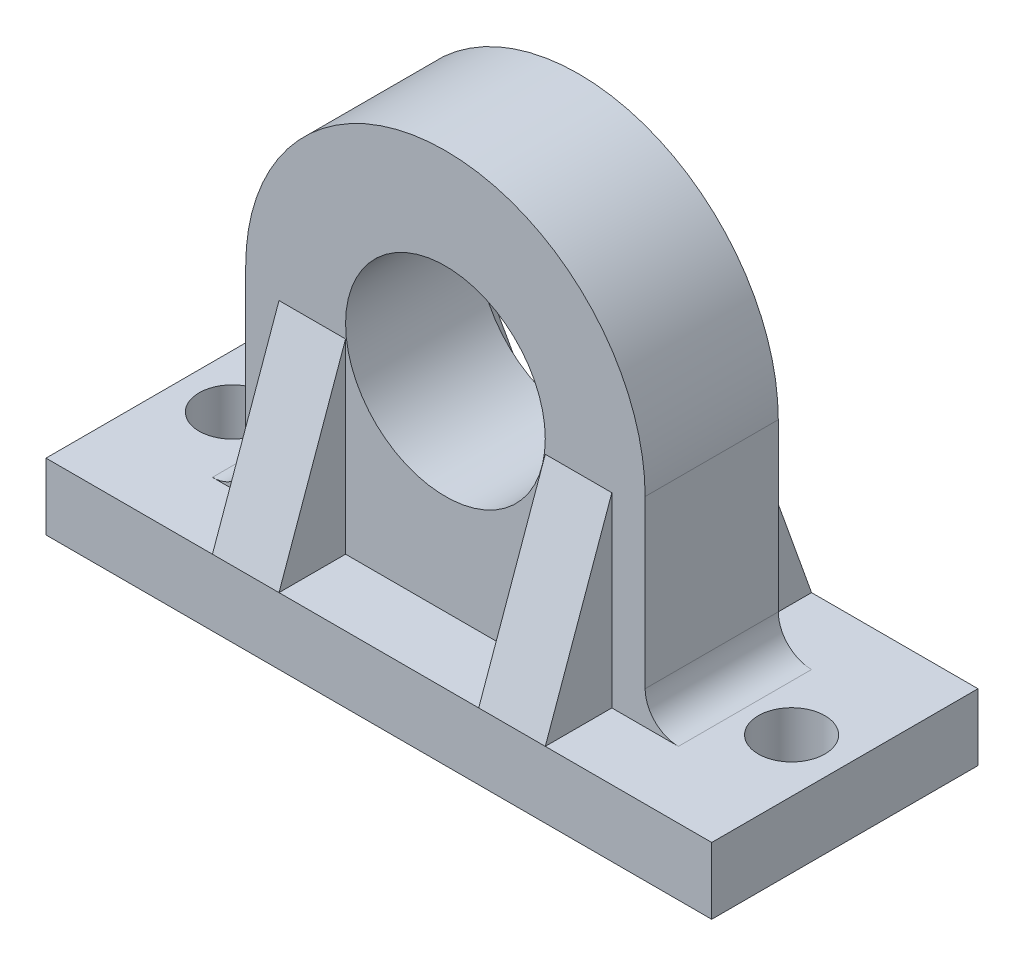
ISO-10303-21;
HEADER;
FILE_DESCRIPTION(('STEP AP214'),'2;1');
FILE_NAME('part.step','',(''),(''),'','','');
FILE_SCHEMA(('AUTOMOTIVE_DESIGN { 1 0 10303 214 1 1 1 1 }'));
ENDSEC;
DATA;
#1=APPLICATION_CONTEXT('core data for automotive mechanical design processes');
#2=APPLICATION_PROTOCOL_DEFINITION('international standard','automotive_design',2000,#1);
#3=PRODUCT_CONTEXT('',#1,'mechanical');
#4=PRODUCT('Part','Part','',(#3));
#5=PRODUCT_RELATED_PRODUCT_CATEGORY('part','',(#4));
#6=PRODUCT_DEFINITION_FORMATION('','',#4);
#7=PRODUCT_DEFINITION_CONTEXT('part definition',#1,'design');
#8=PRODUCT_DEFINITION('design','',#6,#7);
#9=PRODUCT_DEFINITION_SHAPE('','',#8);
#10=(LENGTH_UNIT() NAMED_UNIT(*) SI_UNIT(.MILLI.,.METRE.));
#11=(NAMED_UNIT(*) PLANE_ANGLE_UNIT() SI_UNIT($,.RADIAN.));
#12=(NAMED_UNIT(*) SI_UNIT($,.STERADIAN.) SOLID_ANGLE_UNIT());
#13=UNCERTAINTY_MEASURE_WITH_UNIT(LENGTH_MEASURE(1.E-05),#10,'distance_accuracy_value','');
#14=(GEOMETRIC_REPRESENTATION_CONTEXT(3) GLOBAL_UNCERTAINTY_ASSIGNED_CONTEXT((#13)) GLOBAL_UNIT_ASSIGNED_CONTEXT((#10,
#11,#12)) REPRESENTATION_CONTEXT('',''));
#15=CARTESIAN_POINT('',(0.,0.,0.));
#16=DIRECTION('',(0.,0.,1.));
#17=DIRECTION('',(1.,0.,0.));
#18=AXIS2_PLACEMENT_3D('',#15,#16,#17);
#19=CARTESIAN_POINT('',(0.,10.,20.));
#20=DIRECTION('',(0.,1.,0.));
#21=DIRECTION('',(0.,0.,1.));
#22=AXIS2_PLACEMENT_3D('',#19,#20,#21);
#23=PLANE('',#22);
#24=CARTESIAN_POINT('',(42.,10.,0.));
#25=DIRECTION('',(0.,1.,0.));
#26=DIRECTION('',(0.,0.,1.));
#27=AXIS2_PLACEMENT_3D('',#24,#25,#26);
#28=CIRCLE('',#27,5.);
#29=CARTESIAN_POINT('',(42.,10.,5.));
#30=VERTEX_POINT('',#29);
#31=EDGE_CURVE('E398',#30,#30,#28,.T.);
#32=ORIENTED_EDGE('',*,*,#31,.F.);
#33=EDGE_LOOP('',(#32));
#34=FACE_BOUND('',#33,.T.);
#35=DIRECTION('',(1.,0.,0.));
#36=VECTOR('',#35,1.);
#37=CARTESIAN_POINT('',(0.,10.,10.));
#38=LINE('',#37,#36);
#39=CARTESIAN_POINT('',(25.,10.,10.));
#40=VERTEX_POINT('',#39);
#41=CARTESIAN_POINT('',(35.,10.,10.));
#42=VERTEX_POINT('',#41);
#43=EDGE_CURVE('E217',#40,#42,#38,.T.);
#44=ORIENTED_EDGE('',*,*,#43,.F.);
#45=DIRECTION('',(0.,0.,1.));
#46=VECTOR('',#45,1.);
#47=CARTESIAN_POINT('',(25.,10.,10.));
#48=LINE('',#47,#46);
#49=CARTESIAN_POINT('',(25.,10.,20.));
#50=VERTEX_POINT('',#49);
#51=EDGE_CURVE('E389',#40,#50,#48,.T.);
#52=ORIENTED_EDGE('',*,*,#51,.T.);
#53=DIRECTION('',(1.,0.,0.));
#54=VECTOR('',#53,1.);
#55=CARTESIAN_POINT('',(0.,10.,20.));
#56=LINE('',#55,#54);
#57=CARTESIAN_POINT('',(50.,10.,20.));
#58=VERTEX_POINT('',#57);
#59=EDGE_CURVE('E251',#50,#58,#56,.T.);
#60=ORIENTED_EDGE('',*,*,#59,.T.);
#61=DIRECTION('',(0.,0.,-1.));
#62=VECTOR('',#61,1.);
#63=CARTESIAN_POINT('',(50.,10.,20.));
#64=LINE('',#63,#62);
#65=CARTESIAN_POINT('',(50.,10.,-20.));
#66=VERTEX_POINT('',#65);
#67=EDGE_CURVE('E276',#58,#66,#64,.T.);
#68=ORIENTED_EDGE('',*,*,#67,.T.);
#69=DIRECTION('',(1.,0.,0.));
#70=VECTOR('',#69,1.);
#71=CARTESIAN_POINT('',(0.,10.,-20.));
#72=LINE('',#71,#70);
#73=CARTESIAN_POINT('',(25.,10.,-20.));
#74=VERTEX_POINT('',#73);
#75=EDGE_CURVE('E270',#74,#66,#72,.T.);
#76=ORIENTED_EDGE('',*,*,#75,.F.);
#77=DIRECTION('',(0.,0.,-1.));
#78=VECTOR('',#77,1.);
#79=CARTESIAN_POINT('',(25.,10.,-10.));
#80=LINE('',#79,#78);
#81=CARTESIAN_POINT('',(25.,10.,-10.));
#82=VERTEX_POINT('',#81);
#83=EDGE_CURVE('E335',#82,#74,#80,.T.);
#84=ORIENTED_EDGE('',*,*,#83,.F.);
#85=DIRECTION('',(1.,0.,0.));
#86=VECTOR('',#85,1.);
#87=CARTESIAN_POINT('',(0.,10.,-10.));
#88=LINE('',#87,#86);
#89=CARTESIAN_POINT('',(35.,10.,-10.));
#90=VERTEX_POINT('',#89);
#91=EDGE_CURVE('E232',#82,#90,#88,.T.);
#92=ORIENTED_EDGE('',*,*,#91,.T.);
#93=DIRECTION('',(0.,0.,-1.));
#94=VECTOR('',#93,1.);
#95=CARTESIAN_POINT('',(35.,10.,20.));
#96=LINE('',#95,#94);
#97=EDGE_CURVE('E288',#90,#42,#96,.F.);
#98=ORIENTED_EDGE('',*,*,#97,.T.);
#99=EDGE_LOOP('',(#44,#52,#60,#68,#76,#84,#92,#98));
#100=FACE_BOUND('',#99,.T.);
#101=ADVANCED_FACE('F41',(#34,#100),#23,.T.);
#102=CARTESIAN_POINT('',(0.,0.,10.));
#103=DIRECTION('',(0.,0.,1.));
#104=DIRECTION('',(1.,0.,0.));
#105=AXIS2_PLACEMENT_3D('',#102,#103,#104);
#106=PLANE('',#105);
#107=CARTESIAN_POINT('',(0.,40.,10.));
#108=DIRECTION('',(0.,0.,1.));
#109=DIRECTION('',(1.,0.,0.));
#110=AXIS2_PLACEMENT_3D('',#107,#108,#109);
#111=CIRCLE('',#110,15.);
#112=CARTESIAN_POINT('',(15.,40.,10.));
#113=VERTEX_POINT('',#112);
#114=EDGE_CURVE('E237',#113,#113,#111,.T.);
#115=ORIENTED_EDGE('',*,*,#114,.F.);
#116=EDGE_LOOP('',(#115));
#117=FACE_BOUND('',#116,.T.);
#118=DIRECTION('',(1.,0.,0.));
#119=VECTOR('',#118,1.);
#120=CARTESIAN_POINT('',(15.,38.,10.));
#121=LINE('',#120,#119);
#122=CARTESIAN_POINT('',(15.,38.,10.));
#123=VERTEX_POINT('',#122);
#124=CARTESIAN_POINT('',(25.,38.,10.));
#125=VERTEX_POINT('',#124);
#126=EDGE_CURVE('E379',#123,#125,#121,.T.);
#127=ORIENTED_EDGE('',*,*,#126,.T.);
#128=DIRECTION('',(0.,-1.,0.));
#129=VECTOR('',#128,1.);
#130=CARTESIAN_POINT('',(25.,38.,10.));
#131=LINE('',#130,#129);
#132=EDGE_CURVE('E57',#125,#40,#131,.T.);
#133=ORIENTED_EDGE('',*,*,#132,.T.);
#134=ORIENTED_EDGE('',*,*,#43,.T.);
#135=CARTESIAN_POINT('',(35.,15.,10.));
#136=DIRECTION('',(0.,0.,1.));
#137=DIRECTION('',(1.,0.,0.));
#138=AXIS2_PLACEMENT_3D('',#135,#136,#137);
#139=CIRCLE('',#138,5.);
#140=CARTESIAN_POINT('',(30.,15.,10.));
#141=VERTEX_POINT('',#140);
#142=EDGE_CURVE('E292',#42,#141,#139,.F.);
#143=ORIENTED_EDGE('',*,*,#142,.T.);
#144=DIRECTION('',(0.,1.,0.));
#145=VECTOR('',#144,1.);
#146=CARTESIAN_POINT('',(30.,0.,10.));
#147=LINE('',#146,#145);
#148=CARTESIAN_POINT('',(30.,40.,10.));
#149=VERTEX_POINT('',#148);
#150=EDGE_CURVE('E317',#141,#149,#147,.T.);
#151=ORIENTED_EDGE('',*,*,#150,.T.);
#152=CARTESIAN_POINT('',(0.,40.,10.));
#153=DIRECTION('',(0.,0.,1.));
#154=DIRECTION('',(1.,0.,0.));
#155=AXIS2_PLACEMENT_3D('',#152,#153,#154);
#156=CIRCLE('',#155,30.);
#157=CARTESIAN_POINT('',(-30.,40.,10.));
#158=VERTEX_POINT('',#157);
#159=EDGE_CURVE('E314',#149,#158,#156,.T.);
#160=ORIENTED_EDGE('',*,*,#159,.T.);
#161=DIRECTION('',(0.,1.,0.));
#162=VECTOR('',#161,1.);
#163=CARTESIAN_POINT('',(-30.,0.,10.));
#164=LINE('',#163,#162);
#165=CARTESIAN_POINT('',(-30.,15.,10.));
#166=VERTEX_POINT('',#165);
#167=EDGE_CURVE('E218',#166,#158,#164,.T.);
#168=ORIENTED_EDGE('',*,*,#167,.F.);
#169=CARTESIAN_POINT('',(-35.,15.,10.));
#170=DIRECTION('',(0.,0.,1.));
#171=DIRECTION('',(1.,0.,0.));
#172=AXIS2_PLACEMENT_3D('',#169,#170,#171);
#173=CIRCLE('',#172,5.);
#174=CARTESIAN_POINT('',(-35.,10.,10.));
#175=VERTEX_POINT('',#174);
#176=EDGE_CURVE('E11',#166,#175,#173,.F.);
#177=ORIENTED_EDGE('',*,*,#176,.T.);
#178=CARTESIAN_POINT('',(-25.,10.,10.));
#179=VERTEX_POINT('',#178);
#180=EDGE_CURVE('E212',#175,#179,#38,.T.);
#181=ORIENTED_EDGE('',*,*,#180,.T.);
#182=DIRECTION('',(0.,-1.,0.));
#183=VECTOR('',#182,1.);
#184=CARTESIAN_POINT('',(-25.,38.,10.));
#185=LINE('',#184,#183);
#186=CARTESIAN_POINT('',(-25.,38.,10.));
#187=VERTEX_POINT('',#186);
#188=EDGE_CURVE('E370',#187,#179,#185,.T.);
#189=ORIENTED_EDGE('',*,*,#188,.F.);
#190=DIRECTION('',(-1.,0.,0.));
#191=VECTOR('',#190,1.);
#192=CARTESIAN_POINT('',(-15.,38.,10.));
#193=LINE('',#192,#191);
#194=CARTESIAN_POINT('',(-15.,38.,10.));
#195=VERTEX_POINT('',#194);
#196=EDGE_CURVE('E352',#195,#187,#193,.T.);
#197=ORIENTED_EDGE('',*,*,#196,.F.);
#198=DIRECTION('',(0.,-1.,0.));
#199=VECTOR('',#198,1.);
#200=CARTESIAN_POINT('',(-15.,38.,10.));
#201=LINE('',#200,#199);
#202=CARTESIAN_POINT('',(-15.,10.,10.));
#203=VERTEX_POINT('',#202);
#204=EDGE_CURVE('E213',#195,#203,#201,.T.);
#205=ORIENTED_EDGE('',*,*,#204,.T.);
#206=CARTESIAN_POINT('',(15.,10.,10.));
#207=VERTEX_POINT('',#206);
#208=EDGE_CURVE('E210',#203,#207,#38,.T.);
#209=ORIENTED_EDGE('',*,*,#208,.T.);
#210=DIRECTION('',(0.,-1.,0.));
#211=VECTOR('',#210,1.);
#212=CARTESIAN_POINT('',(15.,38.,10.));
#213=LINE('',#212,#211);
#214=EDGE_CURVE('E191',#123,#207,#213,.T.);
#215=ORIENTED_EDGE('',*,*,#214,.F.);
#216=EDGE_LOOP('',(#127,#133,#134,#143,#151,#160,#168,#177,#181,#189,#197,#205,#209,#215));
#217=FACE_BOUND('',#216,.T.);
#218=ADVANCED_FACE('F211',(#117,#217),#106,.T.);
#219=DIRECTION('',(0.,0.,1.));
#220=VECTOR('',#219,1.);
#221=CARTESIAN_POINT('',(15.,10.,10.));
#222=LINE('',#221,#220);
#223=CARTESIAN_POINT('',(15.,10.,20.));
#224=VERTEX_POINT('',#223);
#225=EDGE_CURVE('E192',#207,#224,#222,.T.);
#226=ORIENTED_EDGE('',*,*,#225,.F.);
#227=ORIENTED_EDGE('',*,*,#208,.F.);
#228=DIRECTION('',(0.,0.,1.));
#229=VECTOR('',#228,1.);
#230=CARTESIAN_POINT('',(-15.,10.,10.));
#231=LINE('',#230,#229);
#232=CARTESIAN_POINT('',(-15.,10.,20.));
#233=VERTEX_POINT('',#232);
#234=EDGE_CURVE('E63',#203,#233,#231,.T.);
#235=ORIENTED_EDGE('',*,*,#234,.T.);
#236=EDGE_CURVE('E209',#233,#224,#56,.T.);
#237=ORIENTED_EDGE('',*,*,#236,.T.);
#238=EDGE_LOOP('',(#226,#227,#235,#237));
#239=FACE_BOUND('',#238,.T.);
#240=ADVANCED_FACE('F207',(#239),#23,.T.);
#241=CARTESIAN_POINT('',(-42.,10.,0.));
#242=DIRECTION('',(0.,1.,0.));
#243=DIRECTION('',(0.,0.,1.));
#244=AXIS2_PLACEMENT_3D('',#241,#242,#243);
#245=CIRCLE('',#244,5.);
#246=CARTESIAN_POINT('',(-42.,10.,5.));
#247=VERTEX_POINT('',#246);
#248=EDGE_CURVE('E388',#247,#247,#245,.F.);
#249=ORIENTED_EDGE('',*,*,#248,.T.);
#250=EDGE_LOOP('',(#249));
#251=FACE_BOUND('',#250,.T.);
#252=DIRECTION('',(0.,0.,1.));
#253=VECTOR('',#252,1.);
#254=CARTESIAN_POINT('',(-25.,10.,10.));
#255=LINE('',#254,#253);
#256=CARTESIAN_POINT('',(-25.,10.,20.));
#257=VERTEX_POINT('',#256);
#258=EDGE_CURVE('E375',#179,#257,#255,.T.);
#259=ORIENTED_EDGE('',*,*,#258,.F.);
#260=ORIENTED_EDGE('',*,*,#180,.F.);
#261=DIRECTION('',(0.,0.,-1.));
#262=VECTOR('',#261,1.);
#263=CARTESIAN_POINT('',(-35.,10.,-10.));
#264=LINE('',#263,#262);
#265=CARTESIAN_POINT('',(-35.,10.,-10.));
#266=VERTEX_POINT('',#265);
#267=EDGE_CURVE('E295',#175,#266,#264,.T.);
#268=ORIENTED_EDGE('',*,*,#267,.T.);
#269=CARTESIAN_POINT('',(-25.,10.,-10.));
#270=VERTEX_POINT('',#269);
#271=EDGE_CURVE('E236',#266,#270,#88,.T.);
#272=ORIENTED_EDGE('',*,*,#271,.T.);
#273=DIRECTION('',(0.,0.,-1.));
#274=VECTOR('',#273,1.);
#275=CARTESIAN_POINT('',(-25.,10.,-10.));
#276=LINE('',#275,#274);
#277=CARTESIAN_POINT('',(-25.,10.,-20.));
#278=VERTEX_POINT('',#277);
#279=EDGE_CURVE('E351',#270,#278,#276,.T.);
#280=ORIENTED_EDGE('',*,*,#279,.T.);
#281=CARTESIAN_POINT('',(-50.,10.,-20.));
#282=VERTEX_POINT('',#281);
#283=EDGE_CURVE('E266',#282,#278,#72,.T.);
#284=ORIENTED_EDGE('',*,*,#283,.F.);
#285=DIRECTION('',(0.,0.,-1.));
#286=VECTOR('',#285,1.);
#287=CARTESIAN_POINT('',(-50.,10.,20.));
#288=LINE('',#287,#286);
#289=CARTESIAN_POINT('',(-50.,10.,20.));
#290=VERTEX_POINT('',#289);
#291=EDGE_CURVE('E273',#290,#282,#288,.T.);
#292=ORIENTED_EDGE('',*,*,#291,.F.);
#293=EDGE_CURVE('E253',#290,#257,#56,.T.);
#294=ORIENTED_EDGE('',*,*,#293,.T.);
#295=EDGE_LOOP('',(#259,#260,#268,#272,#280,#284,#292,#294));
#296=FACE_BOUND('',#295,.T.);
#297=ADVANCED_FACE('F428',(#251,#296),#23,.T.);
#298=CARTESIAN_POINT('',(0.,0.,-10.));
#299=DIRECTION('',(0.,0.,1.));
#300=DIRECTION('',(1.,0.,0.));
#301=AXIS2_PLACEMENT_3D('',#298,#299,#300);
#302=PLANE('',#301);
#303=DIRECTION('',(-1.,0.,0.));
#304=VECTOR('',#303,1.);
#305=CARTESIAN_POINT('',(-15.,38.,-10.));
#306=LINE('',#305,#304);
#307=CARTESIAN_POINT('',(-15.,38.,-10.));
#308=VERTEX_POINT('',#307);
#309=CARTESIAN_POINT('',(-25.,38.,-10.));
#310=VERTEX_POINT('',#309);
#311=EDGE_CURVE('E341',#308,#310,#306,.T.);
#312=ORIENTED_EDGE('',*,*,#311,.T.);
#313=DIRECTION('',(0.,-1.,0.));
#314=VECTOR('',#313,1.);
#315=CARTESIAN_POINT('',(-25.,38.,-10.));
#316=LINE('',#315,#314);
#317=EDGE_CURVE('E353',#310,#270,#316,.T.);
#318=ORIENTED_EDGE('',*,*,#317,.T.);
#319=ORIENTED_EDGE('',*,*,#271,.F.);
#320=CARTESIAN_POINT('',(-35.,15.,-10.));
#321=DIRECTION('',(0.,0.,1.));
#322=DIRECTION('',(1.,0.,0.));
#323=AXIS2_PLACEMENT_3D('',#320,#321,#322);
#324=CIRCLE('',#323,5.);
#325=CARTESIAN_POINT('',(-30.,15.,-10.));
#326=VERTEX_POINT('',#325);
#327=EDGE_CURVE('E47',#266,#326,#324,.T.);
#328=ORIENTED_EDGE('',*,*,#327,.T.);
#329=DIRECTION('',(0.,1.,0.));
#330=VECTOR('',#329,1.);
#331=CARTESIAN_POINT('',(-30.,0.,-10.));
#332=LINE('',#331,#330);
#333=CARTESIAN_POINT('',(-30.,40.,-10.));
#334=VERTEX_POINT('',#333);
#335=EDGE_CURVE('E231',#326,#334,#332,.T.);
#336=ORIENTED_EDGE('',*,*,#335,.T.);
#337=CARTESIAN_POINT('',(0.,40.,-10.));
#338=DIRECTION('',(0.,0.,1.));
#339=DIRECTION('',(1.,0.,0.));
#340=AXIS2_PLACEMENT_3D('',#337,#338,#339);
#341=CIRCLE('',#340,30.);
#342=CARTESIAN_POINT('',(30.,40.,-10.));
#343=VERTEX_POINT('',#342);
#344=EDGE_CURVE('E229',#343,#334,#341,.T.);
#345=ORIENTED_EDGE('',*,*,#344,.F.);
#346=DIRECTION('',(0.,1.,0.));
#347=VECTOR('',#346,1.);
#348=CARTESIAN_POINT('',(30.,0.,-10.));
#349=LINE('',#348,#347);
#350=CARTESIAN_POINT('',(30.,15.,-10.));
#351=VERTEX_POINT('',#350);
#352=EDGE_CURVE('E227',#351,#343,#349,.T.);
#353=ORIENTED_EDGE('',*,*,#352,.F.);
#354=CARTESIAN_POINT('',(35.,15.,-10.));
#355=DIRECTION('',(0.,0.,1.));
#356=DIRECTION('',(1.,0.,0.));
#357=AXIS2_PLACEMENT_3D('',#354,#355,#356);
#358=CIRCLE('',#357,5.);
#359=EDGE_CURVE('E289',#351,#90,#358,.T.);
#360=ORIENTED_EDGE('',*,*,#359,.T.);
#361=ORIENTED_EDGE('',*,*,#91,.F.);
#362=DIRECTION('',(0.,-1.,0.));
#363=VECTOR('',#362,1.);
#364=CARTESIAN_POINT('',(25.,38.,-10.));
#365=LINE('',#364,#363);
#366=CARTESIAN_POINT('',(25.,38.,-10.));
#367=VERTEX_POINT('',#366);
#368=EDGE_CURVE('E327',#367,#82,#365,.T.);
#369=ORIENTED_EDGE('',*,*,#368,.F.);
#370=DIRECTION('',(1.,0.,0.));
#371=VECTOR('',#370,1.);
#372=CARTESIAN_POINT('',(15.,38.,-10.));
#373=LINE('',#372,#371);
#374=CARTESIAN_POINT('',(15.,38.,-10.));
#375=VERTEX_POINT('',#374);
#376=EDGE_CURVE('E226',#375,#367,#373,.T.);
#377=ORIENTED_EDGE('',*,*,#376,.F.);
#378=DIRECTION('',(0.,-1.,0.));
#379=VECTOR('',#378,1.);
#380=CARTESIAN_POINT('',(15.,38.,-10.));
#381=LINE('',#380,#379);
#382=CARTESIAN_POINT('',(15.,10.,-10.));
#383=VERTEX_POINT('',#382);
#384=EDGE_CURVE('E323',#375,#383,#381,.T.);
#385=ORIENTED_EDGE('',*,*,#384,.T.);
#386=CARTESIAN_POINT('',(-15.,10.,-10.));
#387=VERTEX_POINT('',#386);
#388=EDGE_CURVE('E239',#387,#383,#88,.T.);
#389=ORIENTED_EDGE('',*,*,#388,.F.);
#390=DIRECTION('',(0.,-1.,0.));
#391=VECTOR('',#390,1.);
#392=CARTESIAN_POINT('',(-15.,38.,-10.));
#393=LINE('',#392,#391);
#394=EDGE_CURVE('E356',#308,#387,#393,.T.);
#395=ORIENTED_EDGE('',*,*,#394,.F.);
#396=EDGE_LOOP('',(#312,#318,#319,#328,#336,#345,#353,#360,#361,#369,#377,#385,#389,#395));
#397=FACE_BOUND('',#396,.T.);
#398=CARTESIAN_POINT('',(0.,40.,-10.));
#399=DIRECTION('',(0.,0.,1.));
#400=DIRECTION('',(1.,0.,0.));
#401=AXIS2_PLACEMENT_3D('',#398,#399,#400);
#402=CIRCLE('',#401,15.);
#403=CARTESIAN_POINT('',(15.,40.,-10.));
#404=VERTEX_POINT('',#403);
#405=EDGE_CURVE('E224',#404,#404,#402,.T.);
#406=ORIENTED_EDGE('',*,*,#405,.T.);
#407=EDGE_LOOP('',(#406));
#408=FACE_BOUND('',#407,.T.);
#409=ADVANCED_FACE('F301',(#397,#408),#302,.F.);
#410=DIRECTION('',(0.,0.,-1.));
#411=VECTOR('',#410,1.);
#412=CARTESIAN_POINT('',(-15.,10.,-10.));
#413=LINE('',#412,#411);
#414=CARTESIAN_POINT('',(-15.,10.,-20.));
#415=VERTEX_POINT('',#414);
#416=EDGE_CURVE('E348',#387,#415,#413,.T.);
#417=ORIENTED_EDGE('',*,*,#416,.F.);
#418=ORIENTED_EDGE('',*,*,#388,.T.);
#419=DIRECTION('',(0.,0.,-1.));
#420=VECTOR('',#419,1.);
#421=CARTESIAN_POINT('',(15.,10.,-10.));
#422=LINE('',#421,#420);
#423=CARTESIAN_POINT('',(15.,10.,-20.));
#424=VERTEX_POINT('',#423);
#425=EDGE_CURVE('E330',#383,#424,#422,.T.);
#426=ORIENTED_EDGE('',*,*,#425,.T.);
#427=EDGE_CURVE('E272',#415,#424,#72,.T.);
#428=ORIENTED_EDGE('',*,*,#427,.F.);
#429=EDGE_LOOP('',(#417,#418,#426,#428));
#430=FACE_BOUND('',#429,.T.);
#431=ADVANCED_FACE('F408',(#430),#23,.T.);
#432=CARTESIAN_POINT('',(0.,0.,20.));
#433=DIRECTION('',(0.,1.,0.));
#434=DIRECTION('',(0.,0.,1.));
#435=AXIS2_PLACEMENT_3D('',#432,#433,#434);
#436=PLANE('',#435);
#437=CARTESIAN_POINT('',(42.,0.,0.));
#438=DIRECTION('',(0.,-1.,0.));
#439=DIRECTION('',(0.,0.,1.));
#440=AXIS2_PLACEMENT_3D('',#437,#438,#439);
#441=CIRCLE('',#440,5.);
#442=CARTESIAN_POINT('',(42.,0.,5.));
#443=VERTEX_POINT('',#442);
#444=EDGE_CURVE('E399',#443,#443,#441,.T.);
#445=ORIENTED_EDGE('',*,*,#444,.F.);
#446=EDGE_LOOP('',(#445));
#447=FACE_BOUND('',#446,.T.);
#448=CARTESIAN_POINT('',(-42.,0.,0.));
#449=DIRECTION('',(0.,1.,0.));
#450=DIRECTION('',(0.,0.,1.));
#451=AXIS2_PLACEMENT_3D('',#448,#449,#450);
#452=CIRCLE('',#451,5.);
#453=CARTESIAN_POINT('',(-42.,0.,5.));
#454=VERTEX_POINT('',#453);
#455=EDGE_CURVE('E395',#454,#454,#452,.T.);
#456=ORIENTED_EDGE('',*,*,#455,.T.);
#457=EDGE_LOOP('',(#456));
#458=FACE_BOUND('',#457,.T.);
#459=DIRECTION('',(1.,0.,0.));
#460=VECTOR('',#459,1.);
#461=CARTESIAN_POINT('',(0.,0.,-20.));
#462=LINE('',#461,#460);
#463=CARTESIAN_POINT('',(-50.,0.,-20.));
#464=VERTEX_POINT('',#463);
#465=CARTESIAN_POINT('',(50.,0.,-20.));
#466=VERTEX_POINT('',#465);
#467=EDGE_CURVE('E246',#464,#466,#462,.T.);
#468=ORIENTED_EDGE('',*,*,#467,.T.);
#469=DIRECTION('',(0.,0.,-1.));
#470=VECTOR('',#469,1.);
#471=CARTESIAN_POINT('',(50.,0.,20.));
#472=LINE('',#471,#470);
#473=CARTESIAN_POINT('',(50.,0.,20.));
#474=VERTEX_POINT('',#473);
#475=EDGE_CURVE('E277',#474,#466,#472,.T.);
#476=ORIENTED_EDGE('',*,*,#475,.F.);
#477=DIRECTION('',(1.,0.,0.));
#478=VECTOR('',#477,1.);
#479=CARTESIAN_POINT('',(0.,0.,20.));
#480=LINE('',#479,#478);
#481=CARTESIAN_POINT('',(-50.,0.,20.));
#482=VERTEX_POINT('',#481);
#483=EDGE_CURVE('E250',#482,#474,#480,.T.);
#484=ORIENTED_EDGE('',*,*,#483,.F.);
#485=DIRECTION('',(0.,0.,-1.));
#486=VECTOR('',#485,1.);
#487=CARTESIAN_POINT('',(-50.,0.,20.));
#488=LINE('',#487,#486);
#489=EDGE_CURVE('E262',#482,#464,#488,.T.);
#490=ORIENTED_EDGE('',*,*,#489,.T.);
#491=EDGE_LOOP('',(#468,#476,#484,#490));
#492=FACE_BOUND('',#491,.T.);
#493=ADVANCED_FACE('F403',(#447,#458,#492),#436,.F.);
#494=CARTESIAN_POINT('',(50.,0.,20.));
#495=DIRECTION('',(-1.,0.,0.));
#496=DIRECTION('',(0.,0.,1.));
#497=AXIS2_PLACEMENT_3D('',#494,#495,#496);
#498=PLANE('',#497);
#499=DIRECTION('',(0.,1.,0.));
#500=VECTOR('',#499,1.);
#501=CARTESIAN_POINT('',(50.,0.,-20.));
#502=LINE('',#501,#500);
#503=EDGE_CURVE('E261',#466,#66,#502,.T.);
#504=ORIENTED_EDGE('',*,*,#503,.T.);
#505=ORIENTED_EDGE('',*,*,#67,.F.);
#506=DIRECTION('',(0.,1.,0.));
#507=VECTOR('',#506,1.);
#508=CARTESIAN_POINT('',(50.,0.,20.));
#509=LINE('',#508,#507);
#510=EDGE_CURVE('E249',#474,#58,#509,.T.);
#511=ORIENTED_EDGE('',*,*,#510,.F.);
#512=ORIENTED_EDGE('',*,*,#475,.T.);
#513=EDGE_LOOP('',(#504,#505,#511,#512));
#514=FACE_BOUND('',#513,.T.);
#515=ADVANCED_FACE('F410',(#514),#498,.F.);
#516=CARTESIAN_POINT('',(-50.,0.,20.));
#517=DIRECTION('',(-1.,0.,0.));
#518=DIRECTION('',(0.,0.,1.));
#519=AXIS2_PLACEMENT_3D('',#516,#517,#518);
#520=PLANE('',#519);
#521=DIRECTION('',(0.,1.,0.));
#522=VECTOR('',#521,1.);
#523=CARTESIAN_POINT('',(-50.,0.,-20.));
#524=LINE('',#523,#522);
#525=EDGE_CURVE('E252',#464,#282,#524,.T.);
#526=ORIENTED_EDGE('',*,*,#525,.F.);
#527=ORIENTED_EDGE('',*,*,#489,.F.);
#528=DIRECTION('',(0.,1.,0.));
#529=VECTOR('',#528,1.);
#530=CARTESIAN_POINT('',(-50.,0.,20.));
#531=LINE('',#530,#529);
#532=EDGE_CURVE('E260',#482,#290,#531,.T.);
#533=ORIENTED_EDGE('',*,*,#532,.T.);
#534=ORIENTED_EDGE('',*,*,#291,.T.);
#535=EDGE_LOOP('',(#526,#527,#533,#534));
#536=FACE_BOUND('',#535,.T.);
#537=ADVANCED_FACE('F417',(#536),#520,.T.);
#538=CARTESIAN_POINT('',(0.,0.,20.));
#539=DIRECTION('',(0.,0.,1.));
#540=DIRECTION('',(1.,0.,0.));
#541=AXIS2_PLACEMENT_3D('',#538,#539,#540);
#542=PLANE('',#541);
#543=ORIENTED_EDGE('',*,*,#483,.T.);
#544=ORIENTED_EDGE('',*,*,#510,.T.);
#545=ORIENTED_EDGE('',*,*,#59,.F.);
#546=DIRECTION('',(1.,0.,0.));
#547=VECTOR('',#546,1.);
#548=CARTESIAN_POINT('',(15.,10.,20.));
#549=LINE('',#548,#547);
#550=EDGE_CURVE('E374',#224,#50,#549,.T.);
#551=ORIENTED_EDGE('',*,*,#550,.F.);
#552=ORIENTED_EDGE('',*,*,#236,.F.);
#553=DIRECTION('',(-1.,0.,0.));
#554=VECTOR('',#553,1.);
#555=CARTESIAN_POINT('',(-15.,10.,20.));
#556=LINE('',#555,#554);
#557=EDGE_CURVE('E361',#233,#257,#556,.T.);
#558=ORIENTED_EDGE('',*,*,#557,.T.);
#559=ORIENTED_EDGE('',*,*,#293,.F.);
#560=ORIENTED_EDGE('',*,*,#532,.F.);
#561=EDGE_LOOP('',(#543,#544,#545,#551,#552,#558,#559,#560));
#562=FACE_BOUND('',#561,.T.);
#563=ADVANCED_FACE('F551',(#562),#542,.T.);
#564=CARTESIAN_POINT('',(0.,0.,-20.));
#565=DIRECTION('',(0.,0.,1.));
#566=DIRECTION('',(1.,0.,0.));
#567=AXIS2_PLACEMENT_3D('',#564,#565,#566);
#568=PLANE('',#567);
#569=ORIENTED_EDGE('',*,*,#467,.F.);
#570=ORIENTED_EDGE('',*,*,#525,.T.);
#571=ORIENTED_EDGE('',*,*,#283,.T.);
#572=DIRECTION('',(-1.,0.,0.));
#573=VECTOR('',#572,1.);
#574=CARTESIAN_POINT('',(-15.,10.,-20.));
#575=LINE('',#574,#573);
#576=EDGE_CURVE('E332',#415,#278,#575,.T.);
#577=ORIENTED_EDGE('',*,*,#576,.F.);
#578=ORIENTED_EDGE('',*,*,#427,.T.);
#579=DIRECTION('',(1.,0.,0.));
#580=VECTOR('',#579,1.);
#581=CARTESIAN_POINT('',(15.,10.,-20.));
#582=LINE('',#581,#580);
#583=EDGE_CURVE('E324',#424,#74,#582,.T.);
#584=ORIENTED_EDGE('',*,*,#583,.T.);
#585=ORIENTED_EDGE('',*,*,#75,.T.);
#586=ORIENTED_EDGE('',*,*,#503,.F.);
#587=EDGE_LOOP('',(#569,#570,#571,#577,#578,#584,#585,#586));
#588=FACE_BOUND('',#587,.T.);
#589=ADVANCED_FACE('F416',(#588),#568,.F.);
#590=CARTESIAN_POINT('',(30.,0.,10.));
#591=DIRECTION('',(-1.,0.,0.));
#592=DIRECTION('',(0.,0.,1.));
#593=AXIS2_PLACEMENT_3D('',#590,#591,#592);
#594=PLANE('',#593);
#595=ORIENTED_EDGE('',*,*,#150,.F.);
#596=DIRECTION('',(0.,0.,-1.));
#597=VECTOR('',#596,1.);
#598=CARTESIAN_POINT('',(30.,15.,10.));
#599=LINE('',#598,#597);
#600=EDGE_CURVE('E285',#141,#351,#599,.T.);
#601=ORIENTED_EDGE('',*,*,#600,.T.);
#602=ORIENTED_EDGE('',*,*,#352,.T.);
#603=DIRECTION('',(0.,0.,-1.));
#604=VECTOR('',#603,1.);
#605=CARTESIAN_POINT('',(30.,40.,10.));
#606=LINE('',#605,#604);
#607=EDGE_CURVE('E243',#149,#343,#606,.T.);
#608=ORIENTED_EDGE('',*,*,#607,.F.);
#609=EDGE_LOOP('',(#595,#601,#602,#608));
#610=FACE_BOUND('',#609,.T.);
#611=ADVANCED_FACE('F456',(#610),#594,.F.);
#612=CARTESIAN_POINT('',(0.,40.,10.));
#613=DIRECTION('',(0.,0.,-1.));
#614=DIRECTION('',(-1.,0.,0.));
#615=AXIS2_PLACEMENT_3D('',#612,#613,#614);
#616=CYLINDRICAL_SURFACE('',#615,30.);
#617=ORIENTED_EDGE('',*,*,#344,.T.);
#618=DIRECTION('',(0.,0.,-1.));
#619=VECTOR('',#618,1.);
#620=CARTESIAN_POINT('',(-30.,40.,10.));
#621=LINE('',#620,#619);
#622=EDGE_CURVE('E216',#158,#334,#621,.T.);
#623=ORIENTED_EDGE('',*,*,#622,.F.);
#624=ORIENTED_EDGE('',*,*,#159,.F.);
#625=ORIENTED_EDGE('',*,*,#607,.T.);
#626=EDGE_LOOP('',(#617,#623,#624,#625));
#627=FACE_BOUND('',#626,.T.);
#628=ADVANCED_FACE('F463',(#627),#616,.T.);
#629=CARTESIAN_POINT('',(-30.,0.,10.));
#630=DIRECTION('',(-1.,0.,0.));
#631=DIRECTION('',(0.,0.,1.));
#632=AXIS2_PLACEMENT_3D('',#629,#630,#631);
#633=PLANE('',#632);
#634=ORIENTED_EDGE('',*,*,#335,.F.);
#635=DIRECTION('',(0.,0.,-1.));
#636=VECTOR('',#635,1.);
#637=CARTESIAN_POINT('',(-30.,15.,10.));
#638=LINE('',#637,#636);
#639=EDGE_CURVE('E300',#326,#166,#638,.F.);
#640=ORIENTED_EDGE('',*,*,#639,.T.);
#641=ORIENTED_EDGE('',*,*,#167,.T.);
#642=ORIENTED_EDGE('',*,*,#622,.T.);
#643=EDGE_LOOP('',(#634,#640,#641,#642));
#644=FACE_BOUND('',#643,.T.);
#645=ADVANCED_FACE('F308',(#644),#633,.T.);
#646=CARTESIAN_POINT('',(0.,40.,10.));
#647=DIRECTION('',(0.,0.,-1.));
#648=DIRECTION('',(-1.,0.,0.));
#649=AXIS2_PLACEMENT_3D('',#646,#647,#648);
#650=CYLINDRICAL_SURFACE('',#649,15.);
#651=ORIENTED_EDGE('',*,*,#114,.T.);
#652=EDGE_LOOP('',(#651));
#653=FACE_BOUND('',#652,.T.);
#654=ORIENTED_EDGE('',*,*,#405,.F.);
#655=EDGE_LOOP('',(#654));
#656=FACE_BOUND('',#655,.T.);
#657=ADVANCED_FACE('F469',(#653,#656),#650,.F.);
#658=CARTESIAN_POINT('',(35.,15.,10.));
#659=DIRECTION('',(0.,0.,-1.));
#660=DIRECTION('',(-1.,0.,0.));
#661=AXIS2_PLACEMENT_3D('',#658,#659,#660);
#662=CYLINDRICAL_SURFACE('',#661,5.);
#663=ORIENTED_EDGE('',*,*,#142,.F.);
#664=ORIENTED_EDGE('',*,*,#97,.F.);
#665=ORIENTED_EDGE('',*,*,#359,.F.);
#666=ORIENTED_EDGE('',*,*,#600,.F.);
#667=EDGE_LOOP('',(#663,#664,#665,#666));
#668=FACE_BOUND('',#667,.T.);
#669=ADVANCED_FACE('F452',(#668),#662,.F.);
#670=CARTESIAN_POINT('',(-35.,15.,20.));
#671=DIRECTION('',(0.,0.,1.));
#672=DIRECTION('',(1.,0.,0.));
#673=AXIS2_PLACEMENT_3D('',#670,#671,#672);
#674=CYLINDRICAL_SURFACE('',#673,5.);
#675=ORIENTED_EDGE('',*,*,#176,.F.);
#676=ORIENTED_EDGE('',*,*,#639,.F.);
#677=ORIENTED_EDGE('',*,*,#327,.F.);
#678=ORIENTED_EDGE('',*,*,#267,.F.);
#679=EDGE_LOOP('',(#675,#676,#677,#678));
#680=FACE_BOUND('',#679,.T.);
#681=ADVANCED_FACE('F43',(#680),#674,.F.);
#682=CARTESIAN_POINT('',(15.,10.,-20.));
#683=DIRECTION('',(0.,0.336336396998156,-0.941741911594837));
#684=DIRECTION('',(0.,0.941741911594837,0.336336396998156));
#685=AXIS2_PLACEMENT_3D('',#682,#683,#684);
#686=PLANE('',#685);
#687=DIRECTION('',(0.,0.941741911594837,0.336336396998156));
#688=VECTOR('',#687,1.);
#689=CARTESIAN_POINT('',(25.,10.,-20.));
#690=LINE('',#689,#688);
#691=EDGE_CURVE('E326',#74,#367,#690,.T.);
#692=ORIENTED_EDGE('',*,*,#691,.F.);
#693=ORIENTED_EDGE('',*,*,#583,.F.);
#694=DIRECTION('',(0.,0.941741911594837,0.336336396998156));
#695=VECTOR('',#694,1.);
#696=CARTESIAN_POINT('',(15.,10.,-20.));
#697=LINE('',#696,#695);
#698=EDGE_CURVE('E336',#424,#375,#697,.T.);
#699=ORIENTED_EDGE('',*,*,#698,.T.);
#700=ORIENTED_EDGE('',*,*,#376,.T.);
#701=EDGE_LOOP('',(#692,#693,#699,#700));
#702=FACE_BOUND('',#701,.T.);
#703=ADVANCED_FACE('F536',(#702),#686,.T.);
#704=CARTESIAN_POINT('',(15.,0.,0.));
#705=DIRECTION('',(-1.,0.,0.));
#706=DIRECTION('',(0.,0.,1.));
#707=AXIS2_PLACEMENT_3D('',#704,#705,#706);
#708=PLANE('',#707);
#709=ORIENTED_EDGE('',*,*,#425,.F.);
#710=ORIENTED_EDGE('',*,*,#384,.F.);
#711=ORIENTED_EDGE('',*,*,#698,.F.);
#712=EDGE_LOOP('',(#709,#710,#711));
#713=FACE_BOUND('',#712,.T.);
#714=ADVANCED_FACE('F534',(#713),#708,.T.);
#715=CARTESIAN_POINT('',(25.,0.,0.));
#716=DIRECTION('',(-1.,0.,0.));
#717=DIRECTION('',(0.,0.,1.));
#718=AXIS2_PLACEMENT_3D('',#715,#716,#717);
#719=PLANE('',#718);
#720=ORIENTED_EDGE('',*,*,#83,.T.);
#721=ORIENTED_EDGE('',*,*,#691,.T.);
#722=ORIENTED_EDGE('',*,*,#368,.T.);
#723=EDGE_LOOP('',(#720,#721,#722));
#724=FACE_BOUND('',#723,.T.);
#725=ADVANCED_FACE('F531',(#724),#719,.F.);
#726=CARTESIAN_POINT('',(-15.,10.,-20.));
#727=DIRECTION('',(0.,-0.336336396998156,0.941741911594837));
#728=DIRECTION('',(0.,-0.941741911594837,-0.336336396998156));
#729=AXIS2_PLACEMENT_3D('',#726,#727,#728);
#730=PLANE('',#729);
#731=DIRECTION('',(0.,0.941741911594837,0.336336396998156));
#732=VECTOR('',#731,1.);
#733=CARTESIAN_POINT('',(-25.,10.,-20.));
#734=LINE('',#733,#732);
#735=EDGE_CURVE('E349',#278,#310,#734,.T.);
#736=ORIENTED_EDGE('',*,*,#735,.T.);
#737=ORIENTED_EDGE('',*,*,#311,.F.);
#738=DIRECTION('',(0.,0.941741911594837,0.336336396998156));
#739=VECTOR('',#738,1.);
#740=CARTESIAN_POINT('',(-15.,10.,-20.));
#741=LINE('',#740,#739);
#742=EDGE_CURVE('E343',#415,#308,#741,.T.);
#743=ORIENTED_EDGE('',*,*,#742,.F.);
#744=ORIENTED_EDGE('',*,*,#576,.T.);
#745=EDGE_LOOP('',(#736,#737,#743,#744));
#746=FACE_BOUND('',#745,.T.);
#747=ADVANCED_FACE('F436',(#746),#730,.F.);
#748=CARTESIAN_POINT('',(-15.,0.,0.));
#749=DIRECTION('',(1.,0.,0.));
#750=DIRECTION('',(0.,0.,1.));
#751=AXIS2_PLACEMENT_3D('',#748,#749,#750);
#752=PLANE('',#751);
#753=ORIENTED_EDGE('',*,*,#416,.T.);
#754=ORIENTED_EDGE('',*,*,#742,.T.);
#755=ORIENTED_EDGE('',*,*,#394,.T.);
#756=EDGE_LOOP('',(#753,#754,#755));
#757=FACE_BOUND('',#756,.T.);
#758=ADVANCED_FACE('F438',(#757),#752,.T.);
#759=CARTESIAN_POINT('',(-25.,0.,0.));
#760=DIRECTION('',(1.,0.,0.));
#761=DIRECTION('',(0.,0.,1.));
#762=AXIS2_PLACEMENT_3D('',#759,#760,#761);
#763=PLANE('',#762);
#764=ORIENTED_EDGE('',*,*,#279,.F.);
#765=ORIENTED_EDGE('',*,*,#317,.F.);
#766=ORIENTED_EDGE('',*,*,#735,.F.);
#767=EDGE_LOOP('',(#764,#765,#766));
#768=FACE_BOUND('',#767,.T.);
#769=ADVANCED_FACE('F435',(#768),#763,.F.);
#770=CARTESIAN_POINT('',(-15.,10.,20.));
#771=DIRECTION('',(0.,0.336336396998156,0.941741911594837));
#772=DIRECTION('',(0.,-0.941741911594837,0.336336396998156));
#773=AXIS2_PLACEMENT_3D('',#770,#771,#772);
#774=PLANE('',#773);
#775=DIRECTION('',(0.,0.941741911594837,-0.336336396998156));
#776=VECTOR('',#775,1.);
#777=CARTESIAN_POINT('',(-25.,10.,20.));
#778=LINE('',#777,#776);
#779=EDGE_CURVE('E367',#257,#187,#778,.T.);
#780=ORIENTED_EDGE('',*,*,#779,.F.);
#781=ORIENTED_EDGE('',*,*,#557,.F.);
#782=DIRECTION('',(0.,0.941741911594837,-0.336336396998156));
#783=VECTOR('',#782,1.);
#784=CARTESIAN_POINT('',(-15.,10.,20.));
#785=LINE('',#784,#783);
#786=EDGE_CURVE('E380',#233,#195,#785,.T.);
#787=ORIENTED_EDGE('',*,*,#786,.T.);
#788=ORIENTED_EDGE('',*,*,#196,.T.);
#789=EDGE_LOOP('',(#780,#781,#787,#788));
#790=FACE_BOUND('',#789,.T.);
#791=ADVANCED_FACE('F517',(#790),#774,.T.);
#792=CARTESIAN_POINT('',(-15.,0.,0.));
#793=DIRECTION('',(1.,0.,0.));
#794=DIRECTION('',(0.,0.,-1.));
#795=AXIS2_PLACEMENT_3D('',#792,#793,#794);
#796=PLANE('',#795);
#797=ORIENTED_EDGE('',*,*,#234,.F.);
#798=ORIENTED_EDGE('',*,*,#204,.F.);
#799=ORIENTED_EDGE('',*,*,#786,.F.);
#800=EDGE_LOOP('',(#797,#798,#799));
#801=FACE_BOUND('',#800,.T.);
#802=ADVANCED_FACE('F516',(#801),#796,.T.);
#803=CARTESIAN_POINT('',(-25.,0.,0.));
#804=DIRECTION('',(1.,0.,0.));
#805=DIRECTION('',(0.,0.,-1.));
#806=AXIS2_PLACEMENT_3D('',#803,#804,#805);
#807=PLANE('',#806);
#808=ORIENTED_EDGE('',*,*,#258,.T.);
#809=ORIENTED_EDGE('',*,*,#779,.T.);
#810=ORIENTED_EDGE('',*,*,#188,.T.);
#811=EDGE_LOOP('',(#808,#809,#810));
#812=FACE_BOUND('',#811,.T.);
#813=ADVANCED_FACE('F513',(#812),#807,.F.);
#814=CARTESIAN_POINT('',(15.,10.,20.));
#815=DIRECTION('',(0.,-0.336336396998156,-0.941741911594837));
#816=DIRECTION('',(0.,0.941741911594837,-0.336336396998156));
#817=AXIS2_PLACEMENT_3D('',#814,#815,#816);
#818=PLANE('',#817);
#819=DIRECTION('',(0.,0.941741911594837,-0.336336396998156));
#820=VECTOR('',#819,1.);
#821=CARTESIAN_POINT('',(25.,10.,20.));
#822=LINE('',#821,#820);
#823=EDGE_CURVE('E208',#50,#125,#822,.T.);
#824=ORIENTED_EDGE('',*,*,#823,.T.);
#825=ORIENTED_EDGE('',*,*,#126,.F.);
#826=DIRECTION('',(0.,0.941741911594837,-0.336336396998156));
#827=VECTOR('',#826,1.);
#828=CARTESIAN_POINT('',(15.,10.,20.));
#829=LINE('',#828,#827);
#830=EDGE_CURVE('E199',#224,#123,#829,.T.);
#831=ORIENTED_EDGE('',*,*,#830,.F.);
#832=ORIENTED_EDGE('',*,*,#550,.T.);
#833=EDGE_LOOP('',(#824,#825,#831,#832));
#834=FACE_BOUND('',#833,.T.);
#835=ADVANCED_FACE('F512',(#834),#818,.F.);
#836=CARTESIAN_POINT('',(15.,0.,0.));
#837=DIRECTION('',(-1.,0.,0.));
#838=DIRECTION('',(0.,0.,-1.));
#839=AXIS2_PLACEMENT_3D('',#836,#837,#838);
#840=PLANE('',#839);
#841=ORIENTED_EDGE('',*,*,#225,.T.);
#842=ORIENTED_EDGE('',*,*,#830,.T.);
#843=ORIENTED_EDGE('',*,*,#214,.T.);
#844=EDGE_LOOP('',(#841,#842,#843));
#845=FACE_BOUND('',#844,.T.);
#846=ADVANCED_FACE('F193',(#845),#840,.T.);
#847=CARTESIAN_POINT('',(25.,0.,0.));
#848=DIRECTION('',(-1.,0.,0.));
#849=DIRECTION('',(0.,0.,-1.));
#850=AXIS2_PLACEMENT_3D('',#847,#848,#849);
#851=PLANE('',#850);
#852=ORIENTED_EDGE('',*,*,#51,.F.);
#853=ORIENTED_EDGE('',*,*,#132,.F.);
#854=ORIENTED_EDGE('',*,*,#823,.F.);
#855=EDGE_LOOP('',(#852,#853,#854));
#856=FACE_BOUND('',#855,.T.);
#857=ADVANCED_FACE('F501',(#856),#851,.F.);
#858=CARTESIAN_POINT('',(-42.,70.,0.));
#859=DIRECTION('',(0.,-1.,0.));
#860=DIRECTION('',(0.,0.,-1.));
#861=AXIS2_PLACEMENT_3D('',#858,#859,#860);
#862=CYLINDRICAL_SURFACE('',#861,5.);
#863=ORIENTED_EDGE('',*,*,#248,.F.);
#864=EDGE_LOOP('',(#863));
#865=FACE_BOUND('',#864,.T.);
#866=ORIENTED_EDGE('',*,*,#455,.F.);
#867=EDGE_LOOP('',(#866));
#868=FACE_BOUND('',#867,.T.);
#869=ADVANCED_FACE('F497',(#865,#868),#862,.F.);
#870=CARTESIAN_POINT('',(42.,70.,0.));
#871=DIRECTION('',(0.,-1.,0.));
#872=DIRECTION('',(0.,0.,-1.));
#873=AXIS2_PLACEMENT_3D('',#870,#871,#872);
#874=CYLINDRICAL_SURFACE('',#873,5.);
#875=ORIENTED_EDGE('',*,*,#31,.T.);
#876=EDGE_LOOP('',(#875));
#877=FACE_BOUND('',#876,.T.);
#878=ORIENTED_EDGE('',*,*,#444,.T.);
#879=EDGE_LOOP('',(#878));
#880=FACE_BOUND('',#879,.T.);
#881=ADVANCED_FACE('F401',(#877,#880),#874,.F.);
#882=CLOSED_SHELL('',(#101,#218,#240,#297,#409,#431,#493,#515,#537,#563,#589,#611,#628,#645,
#657,#669,#681,#703,#714,#725,#747,#758,#769,#791,#802,#813,#835,#846,#857,#869,#881));
#883=MANIFOLD_SOLID_BREP('B2',#882);
#884=ADVANCED_BREP_SHAPE_REPRESENTATION('',(#18,#883),#14);
#885=SHAPE_DEFINITION_REPRESENTATION(#9,#884);
ENDSEC;
END-ISO-10303-21;
